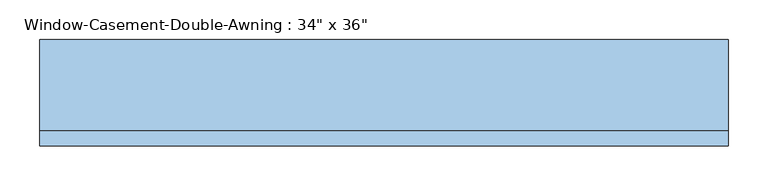
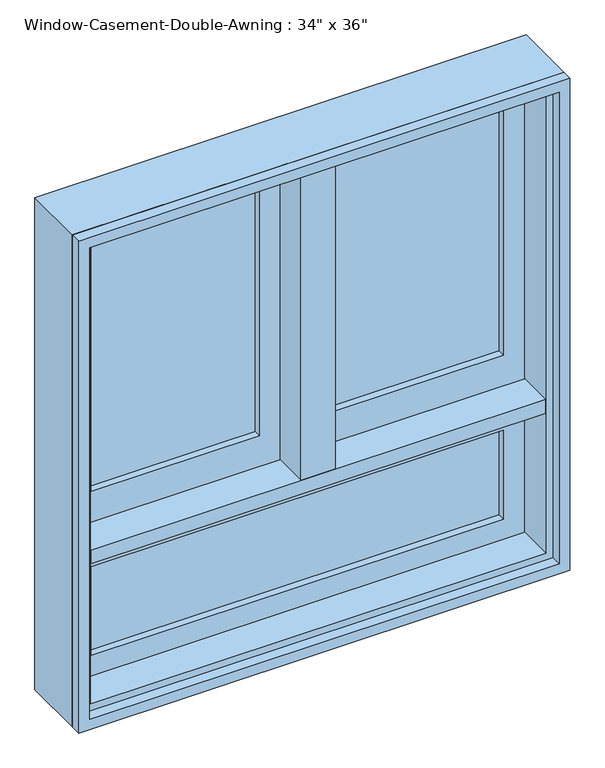
"""IFC4 building model written with IfcOpenShell, lengths in millimetres: window geometry."""

from ifc_helpers import new_model, si_unit, frame, origin, place, context, project, spatial, polyline, outline, extrude, faceted_brep, source, transform, mapped, element, save


def window_622386c7(model_context):
    return source(origin(), model_context, "Body", "SolidModel", [
        faceted_brep([(400.05, 25.4, 1797.05), (400.05, -38.1, 1797.05), (-400.05, -38.1, 1797.05), (-400.05, 25.4, 1797.05), (419.1, 76.2, 1816.1), (419.1, 25.4, 1816.1), (-419.1, 25.4, 1816.1), (-419.1, 76.2, 1816.1), (431.8, -38.1, 1828.8), (431.8, 76.2, 1828.8), (-431.8, 76.2, 1828.8), (-431.8, -38.1, 1828.8), (-400.05, -38.1, 946.15), (-400.05, 25.4, 946.15), (-419.1, 25.4, 927.1), (-419.1, 76.2, 927.1), (-431.8, 76.2, 914.4), (-431.8, -38.1, 914.4), (400.05, -38.1, 946.15), (400.05, 25.4, 946.15), (419.1, 25.4, 927.1), (419.1, 76.2, 927.1), (431.8, 76.2, 914.4), (431.8, -38.1, 914.4)], [[[0, 1, 2, 3]], [[4, 5, 6, 7]], [[8, 9, 10, 11]], [[3, 2, 12, 13]], [[7, 6, 14, 15]], [[11, 10, 16, 17]], [[13, 12, 18, 19]], [[15, 14, 20, 21]], [[17, 16, 22, 23]], [[11, 17, 23, 8], [1, 18, 12, 2]], [[19, 18, 1, 0]], [[5, 20, 14, 6], [3, 13, 19, 0]], [[21, 20, 5, 4]], [[23, 22, 9, 8]], [[9, 22, 16, 10], [7, 15, 21, 4]]]),
        extrude(outline(polyline([(1231.9, 419.1), (1816.1, 419.1), (1816.1, 9.525), (1231.9, 9.525), (1231.9, 419.1)]), holes=[polyline([(1289.05, 66.675), (1758.95, 66.675), (1758.95, 361.95), (1289.05, 361.95), (1289.05, 66.675)])]), frame((0.0, 25.4, 0.0), z_axis=(0.0, 1.0, 0.0), x_axis=(0.0, 0.0, 1.0)), (0.0, 0.0, 1.0), 44.45),
        extrude(outline(polyline([(1816.1, -419.1), (1231.9, -419.1), (1231.9, -9.525), (1816.1, -9.525), (1816.1, -419.1)]), holes=[polyline([(1758.95, -66.675), (1289.05, -66.675), (1289.05, -361.95), (1758.95, -361.95), (1758.95, -66.675)])]), frame((0.0, 25.4, 0.0), z_axis=(0.0, 1.0, 0.0), x_axis=(0.0, 0.0, 1.0)), (0.0, 0.0, 1.0), 44.45),
        extrude(outline(polyline([(361.95, 57.15), (361.95, 50.8), (66.675, 50.8), (66.675, 57.15), (361.95, 57.15)])), frame((0.0, 0.0, 1289.05), z_axis=(0.0, 0.0, 1.0), x_axis=(1.0, 0.0, 0.0)), (0.0, 0.0, 1.0), 469.9),
        extrude(outline(polyline([(66.675, 38.1), (66.675, 44.45), (361.95, 44.45), (361.95, 38.1), (66.675, 38.1)])), frame((0.0, 0.0, 1289.05), z_axis=(0.0, 0.0, 1.0), x_axis=(1.0, 0.0, 0.0)), (0.0, 0.0, 1.0), 469.9),
        extrude(outline(polyline([(-66.675, 57.15), (-66.675, 50.8), (-361.95, 50.8), (-361.95, 57.15), (-66.675, 57.15)])), frame((0.0, 0.0, 1289.05), z_axis=(0.0, 0.0, 1.0), x_axis=(1.0, 0.0, 0.0)), (0.0, 0.0, 1.0), 469.9),
        extrude(outline(polyline([(-361.95, 38.1), (-361.95, 44.45), (-66.675, 44.45), (-66.675, 38.1), (-361.95, 38.1)])), frame((0.0, 0.0, 1289.05), z_axis=(0.0, 0.0, 1.0), x_axis=(1.0, 0.0, 0.0)), (0.0, 0.0, 1.0), 469.9),
        extrude(outline(polyline([(400.05, -38.1), (-400.05, -38.1), (-400.05, 25.4), (-419.1, 25.4), (-419.1, 76.2), (419.1, 76.2), (419.1, 25.4), (400.05, 25.4), (400.05, -38.1)])), frame((0.0, 0.0, 1206.5), z_axis=(0.0, 0.0, 1.0), x_axis=(1.0, 0.0, 0.0)), (0.0, 0.0, 1.0), 25.4),
        extrude(outline(polyline([(1206.5, -419.1), (927.1, -419.1), (927.1, 419.1), (1206.5, 419.1), (1206.5, -419.1)]), holes=[polyline([(1149.35, 361.95), (984.25, 361.95), (984.25, -361.95), (1149.35, -361.95), (1149.35, 361.95)])]), frame((0.0, 25.4, 0.0), z_axis=(0.0, 1.0, 0.0), x_axis=(0.0, 0.0, 1.0)), (0.0, 0.0, 1.0), 44.45),
        extrude(outline(polyline([(361.95, 57.15), (361.95, 50.8), (-361.95, 50.8), (-361.95, 57.15), (361.95, 57.15)])), frame((0.0, 0.0, 984.25), z_axis=(0.0, 0.0, 1.0), x_axis=(1.0, 0.0, 0.0)), (0.0, 0.0, 1.0), 165.1),
        extrude(outline(polyline([(361.95, 44.45), (361.95, 38.1), (-361.95, 38.1), (-361.95, 44.45), (361.95, 44.45)])), frame((0.0, 0.0, 984.25), z_axis=(0.0, 0.0, 1.0), x_axis=(1.0, 0.0, 0.0)), (0.0, 0.0, 1.0), 165.1),
        extrude(outline(polyline([(1828.8, -431.8), (914.4, -431.8), (914.4, 431.8), (1828.8, 431.8), (1828.8, -431.8)]), holes=[polyline([(1809.75, 412.75), (933.45, 412.75), (933.45, -412.75), (1809.75, -412.75), (1809.75, 412.75)])]), frame((0.0, -57.15, 0.0), z_axis=(0.0, 1.0, 0.0), x_axis=(0.0, 0.0, 1.0)), (0.0, 0.0, 1.0), 19.05),
        faceted_brep([(9.525, 76.2, 1816.1), (-9.525, 76.2, 1816.1), (-9.525, 25.4, 1816.1), (9.525, 25.4, 1816.1), (9.525, 76.2, 1231.9), (9.525, 25.4, 1231.9), (30.1625, 25.4, 1231.9), (30.1625, -38.1, 1231.9), (-30.1625, -38.1, 1231.9), (-30.1625, 25.4, 1231.9), (-9.525, 25.4, 1231.9), (-9.525, 76.2, 1231.9), (-9.525, 25.4, 1797.05), (-30.1625, 25.4, 1797.05), (-30.1625, -38.1, 1797.05), (30.1625, -38.1, 1797.05), (30.1625, 25.4, 1797.05), (9.525, 25.4, 1797.05)], [[[0, 1, 2, 3]], [[4, 5, 6, 7, 8, 9, 10, 11]], [[1, 0, 4, 11]], [[2, 1, 11, 10, 12]], [[10, 9, 13, 12]], [[9, 8, 14, 13]], [[8, 7, 15, 14]], [[7, 6, 16, 15]], [[6, 5, 17, 16]], [[0, 3, 17, 5, 4]], [[12, 17, 3, 2]], [[17, 12, 13, 14, 15, 16]]]),
    ])


if __name__ == "__main__":
    model = new_model("IFC4")
    model_context = context("Model", 3, world=origin())
    ifc_project = project(units=[si_unit("LENGTHUNIT", "METRE", prefix="MILLI")], contexts=[model_context])
    site = spatial("IfcSite", under=ifc_project)
    building = spatial("IfcBuilding", under=site)
    placement = place(None, origin())
    window_shape = window_622386c7(model_context)
    element("IfcWindow", 1, ObjectType="Window-Casement-Double-Awning : 34\" x 36\"", at=placement, inside=building, context=model_context, shape_type="MappedRepresentation", body=[
        mapped(window_shape, transform((0.0, 0.0, 0.0), x_axis=(1.0, 0.0, 0.0), y_axis=(0.0, 1.0, 0.0), z_axis=(0.0, 0.0, 1.0))),
    ])
    save(model, "model.ifc")

# Revit data of these elements
# Type "Window-Casement-Double-Awning : 34\" x 36\""
#   Type Mark = "28"
#   Fire Rating = "0.5h"
#   Assembly Code = "B2020100"
#   Analytic Construction = "Double glazing - domestic"
#   Window Inset [instance default] = 0' - 0"
#   Wall Thickness [instance default] = 0' - 6"
#   Interior Wall Closure [instance default] = 0' - 2 1/4"
#   Half Width = 1' - 5"
#   Visual Light Transmittance = 0.81
#   Thermal Resistance (R) = 1.8146 (h·ft²·°F)/BTU
#   Solar Heat Gain Coefficient = 0.76
#   Rough Width = 2' - 10 1/2"
#   Rough Height = 3' - 0 1/2"
#   Open Window Height = 2' - 0"
#   Height = 3' - 0"
#   Heat Transfer Coefficient (U) = 0.5511 BTU/(h·ft²·°F)
#   Frame Extension [instance default] = 0' - 0 1/4"
#   Exterior Wall Closure [instance default] = 0' - 1 1/4"
#   Awning Height = 1' - 0"
#   Extension Jamb [instance default] = 0' - 2 1/4"
#   Default Sill Height = 3' - 0"
#   Width = 2' - 10"
#   Top Muntin Visibility = yes
#   Interior Trim Visibility [instance default] = yes
#   Bottom Muntin Visibility = yes
#   Exterior Trim Visibility [instance default] = yes
#   Extension Jamb Visibility [instance default] = yes
#   Interior Trim Material = Wood - Stained
#   Muntin Pattern = Muntin Pattern_2x2 : Muntin Pattern_2x2
#   Interior Trim = Trim-Window-Interior-Flat : Picture Frame
#   Interior Frame Material = Wood - Stained
#   Exterior Trim Material = Clad - White
#   Glass Panel Material = Glass
#   Exterior Trim = Trim-Window-Exterior-Flat : with Sill
#   Exterior Frame Material = Clad - White
#   Wall Closure = (empty or 0)
# Element 1 (IfcWindow, "Window-Casement-Double-Awning : 34\" x 36\"")
#   Wall Thickness = 0' - 4 1/2"
#   Extension Jamb = 0' - 0 3/4"
#   Materials on its faces: "Wood - Stained", "Glass", "Clad - White"
# Materials
#   "Wood - Stained": class "Wood", colour RGB 224 178 126, transparency 0, Cost = 0
#   "Clad - White": class "Wood", colour RGB 242 242 238, transparency 0, Cost = 0
#   "Glass": class "Glass", colour RGB 0 128 192, transparency 0.75, Description = "Soda Lime Glass", Cost = 0
